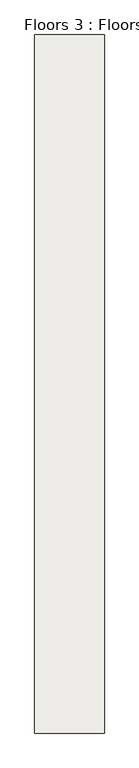
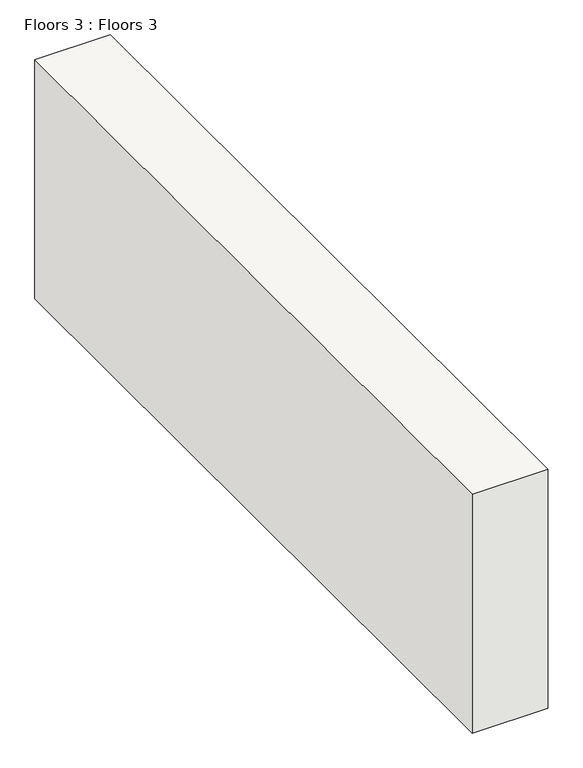
"""IFC4 building model written with IfcOpenShell, lengths in millimetres: slab geometry, Floors 3 : Floors 3."""

from ifc_helpers import new_model, si_unit, frame, origin, place, context, project, spatial, polyline, outline, extrude, source, transform, mapped, element, save


def floors_3_floors_3_f25fb9f3(model_context):
    return source(origin(), model_context, "Body", "SweptSolid", [
        extrude(outline(polyline([(-22.6504261, -2222.8464178), (-205.0528935, -2222.8464178), (-205.0528935, -394.0464931), (-22.6504261, -394.0464931), (-22.6504261, -2222.8464178)])), frame((0.0, 0.0, 5486.4), z_axis=(0.0, 0.0, 1.0), x_axis=(1.0, 0.0, 0.0)), (0.0, 0.0, 1.0), 609.6),
    ])


if __name__ == "__main__":
    model = new_model("IFC4")
    model_context = context("Model", 3, world=origin())
    ifc_project = project(units=[si_unit("LENGTHUNIT", "METRE", prefix="MILLI")], contexts=[model_context])
    site = spatial("IfcSite", under=ifc_project)
    building = spatial("IfcBuilding", under=site)
    placement = place(None, origin())
    floors_3_floors_3_shape = floors_3_floors_3_f25fb9f3(model_context)
    element("IfcSlab", 1, ObjectType="Floors 3 : Floors 3", at=placement, inside=building, context=model_context, shape_type="MappedRepresentation", body=[
        mapped(floors_3_floors_3_shape, transform((0.0, 0.0, 0.0), x_axis=(1.0, 0.0, 0.0), y_axis=(0.0, 1.0, 0.0), z_axis=(0.0, 0.0, 1.0))),
    ])
    save(model, "model.ifc")

# Revit data of these elements
# Element 1 (IfcSlab, "Floors 3 : Floors 3")
#   Materials on its faces: "Default Floor"
# Materials
#   "Default Floor": colour RGB 128 128 128, transparency 0, Cost = 0
